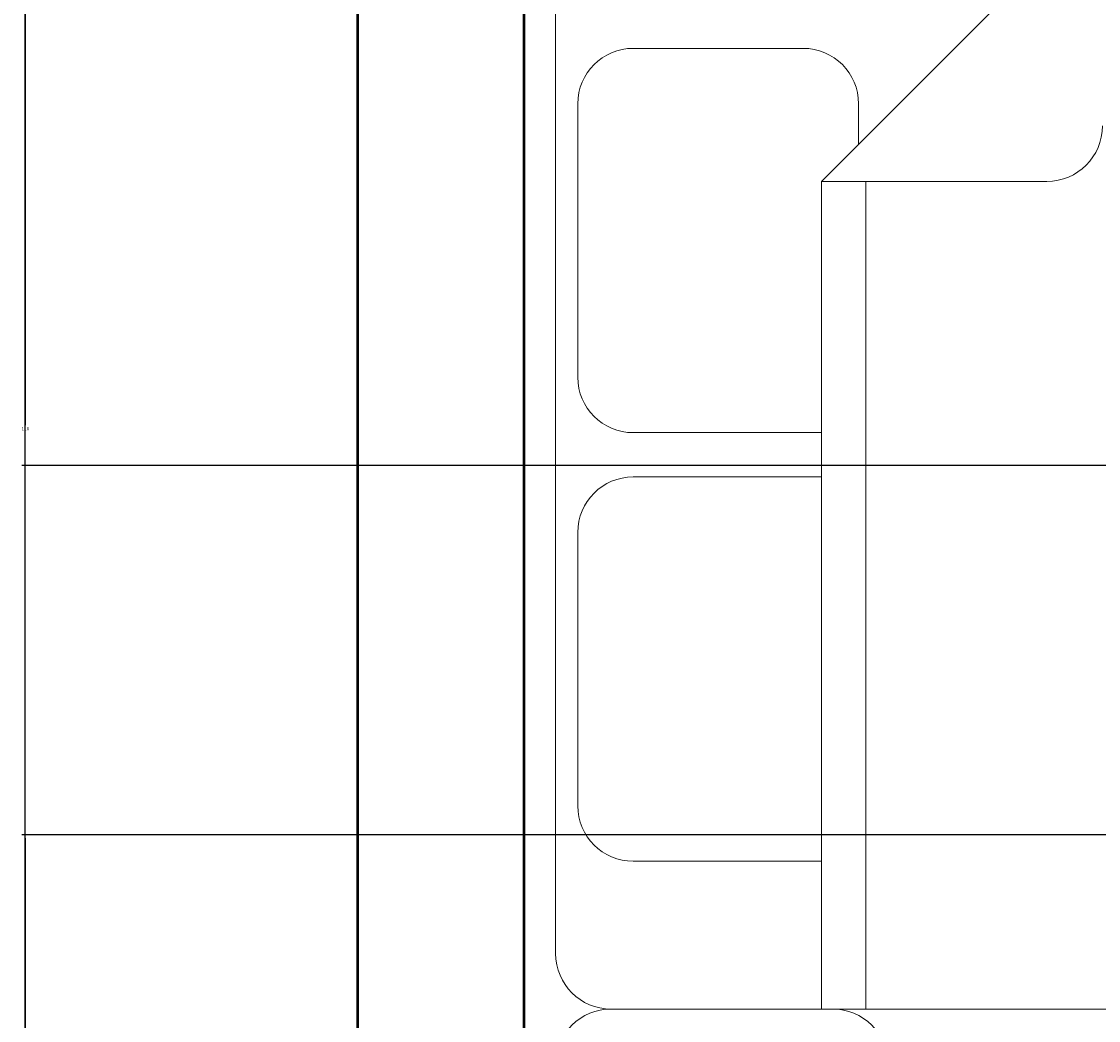
# Model space of a CAD drawing. Units: inches. Extents: x 2621 to 2849, y 2066 to 2463.
# Tile 14 of 28: x 2621 to 2679, y 2345 to 2399. Entities that reach past the tile are written whole.
import ezdxf

# ---------------------------------------------------------------- set-up
doc = ezdxf.new("R2010")
doc.units = ezdxf.units.IN
for name, color, linetype, lineweight in [('A-ANNO-DIMS', 2, 'Continuous', 18), ('A-FURN', 8, 'Continuous', 18), ('A-WALL', 7, 'Continuous', 50)]:
    doc.layers.add(name, color=color, linetype=linetype, lineweight=lineweight)
doc.styles.get("Standard").update_dxf_attribs({"font": 'arial.ttf'})
doc.dimstyles.get("Standard").update_dxf_attribs({"dimtxt": 0.18, "dimasz": 0.18, "dimexe": 0.18, "dimexo": 0.0625, "dimgap": 0.09, "dimtad": 0, "dimtih": 1, "dimtoh": 1, "dimdec": 4, "dimzin": 0, "dimdsep": 46, "dimtxsty": 'Standard', "dimcen": 0.09, "dimadec": 0, "dimazin": 0, "dimtfac": 1, "dimtdec": 4, "dimtofl": 0, "dimtmove": 0, "dimatfit": 3, "dimfxl": 1, "dimtolj": 1, "dimtzin": 0, "dimarcsym": 0})

# ---------------------------------------------------------------- blocks, each defined once
blk = doc.blocks.new('Bed - Queen')
for p, q in [((3, 0), (56.99999, 0)), ((10.99999, -1.2), (25.79998, -1.2)), ((34.19999, -1.2), (48.99999, -1.2)), ((0, -77.00003), (0, -3)), ((7.99999, -14.4), (7.99999, -4.2)), ((28.79998, -4.2), (28.79998, -14.4)), ((31.19999, -14.4), (31.19999, -4.2)), ((51.99999, -4.2), (51.99999, -13.4)), ((0, -14.4), (44.8, -14.4)), ((59.99999, -29.6), (44.8, -14.4)), ((44.8, -14.4), (44.8, -26.6)), ((44.8, -16.8), (0, -16.8)), ((48.99999, -16.4), (46.79936, -16.4))]:
    blk.add_line(p, q)
for centre, start, end in [((3, -3), 90, 180), ((10.99999, -4.2), 90, 180), ((25.79998, -4.2), 0, 90), ((34.19999, -4.2), 90, 180), ((48.99999, -4.2), 0, 90), ((48.99999, -13.4), 270, 0), ((47.8, -26.6), 180, 270)]:
    blk.add_arc(centre, 3, start, end)
blk = doc.blocks.new('*D46')
at = {"layer": 'A-ANNO-DIMS', "color": 0, "lineweight": -2, "transparency": 16777216}
for p, q in [((2647.808, 2435.375), (2620.687, 2435.375)), ((2620.867, 2435.195), (2620.867, 2377.556)), ((2620.867, 2319.555), (2620.867, 2377.193)), ((2647.808, 2319.375), (2620.687, 2319.375))]:
    blk.add_line(p, q, dxfattribs=at)
at = {"layer": 'A-ANNO-DIMS', "color": 0, "transparency": 16777216}
for points in [[(2620.837, 2435.195), (2620.897, 2435.195), (2620.867, 2435.375)], [(2620.837, 2319.555), (2620.897, 2319.555), (2620.867, 2319.375)]]:
    blk.add_solid(points, dxfattribs=at)
at = {"layer": 'Defpoints', "color": 0, "transparency": 16777216}
for p in [(2620.867, 2435.375), (2647.87, 2435.375), (2647.87, 2319.375)]:
    blk.add_point(p, dxfattribs=at)
at = {"layer": 'A-ANNO-DIMS', "color": 0, "transparency": 16777216, "insert": (2620.867, 2377.375), "char_height": 0.18, "attachment_point": 5}
blk.add_mtext('\\A1;116', dxfattribs=at)
blk = doc.blocks.new('*D50')
at = {"layer": 'A-ANNO-DIMS', "color": 0, "lineweight": -2, "transparency": 16777216}
for p, q in [((2763.808, 2355.375), (2620.687, 2355.375)), ((2620.867, 2355.195), (2620.867, 2340.557)), ((2620.867, 2325.555), (2620.867, 2340.193)), ((2763.808, 2325.375), (2620.687, 2325.375))]:
    blk.add_line(p, q, dxfattribs=at)
at = {"layer": 'A-ANNO-DIMS', "color": 0, "transparency": 16777216}
for points in [[(2620.837, 2355.195), (2620.897, 2355.195), (2620.867, 2355.375)], [(2620.837, 2325.555), (2620.897, 2325.555), (2620.867, 2325.375)]]:
    blk.add_solid(points, dxfattribs=at)
at = {"layer": 'Defpoints', "color": 0, "transparency": 16777216}
for p in [(2620.867, 2355.375), (2763.87, 2355.375), (2763.87, 2325.375)]:
    blk.add_point(p, dxfattribs=at)
at = {"layer": 'A-ANNO-DIMS', "color": 0, "transparency": 16777216, "insert": (2620.867, 2340.375), "char_height": 0.18, "attachment_point": 5}
blk.add_mtext('\\A1;30', dxfattribs=at)
blk = doc.blocks.new('*D68')
at = {"layer": 'A-ANNO-DIMS', "color": 0, "lineweight": -2, "transparency": 16777216}
for p, q in [((2745.808, 2435.375), (2620.687, 2435.375)), ((2620.867, 2435.195), (2620.867, 2405.556)), ((2620.867, 2375.555), (2620.867, 2405.193)), ((2745.808, 2375.375), (2620.687, 2375.375))]:
    blk.add_line(p, q, dxfattribs=at)
at = {"layer": 'A-ANNO-DIMS', "color": 0, "transparency": 16777216}
for points in [[(2620.837, 2435.195), (2620.897, 2435.195), (2620.867, 2435.375)], [(2620.837, 2375.555), (2620.897, 2375.555), (2620.867, 2375.375)]]:
    blk.add_solid(points, dxfattribs=at)
at = {"layer": 'Defpoints', "color": 0, "transparency": 16777216}
for p in [(2620.867, 2435.375), (2745.87, 2435.375), (2745.87, 2375.375)]:
    blk.add_point(p, dxfattribs=at)
at = {"layer": 'A-ANNO-DIMS', "color": 0, "transparency": 16777216, "insert": (2620.867, 2405.375), "char_height": 0.18, "attachment_point": 5}
blk.add_mtext('\\A1;60', dxfattribs=at)

msp = doc.modelspace()

# ---------------------------------------------------------------- linework, layer by layer
at = {"layer": 'A-FURN'}
msp.add_lwpolyline([(2652.5811, 2327.9537), (2664.5811, 2327.9537, 0.4142136), (2667.5811, 2330.9537), (2667.5811, 2342.9537, 0.4142136), (2664.5811, 2345.9537), (2652.5811, 2345.9537, 0.4142136), (2649.5811, 2342.9537), (2649.5811, 2330.9537, 0.4142136)], format="xyb", close=True, dxfattribs=at)
at = {"layer": 'A-WALL'}
msp.add_line((2647.8701, 2319.3746), (2647.8701, 2435.3746), dxfattribs=at)
msp.add_lwpolyline([(2761.8701, 2084.3746), (2638.8701, 2084.3746), (2638.8701, 2444.3746), (2830.8701, 2444.3746), (2830.8701, 2084.3746), (2797.8701, 2084.3746)], dxfattribs=at)

# ---------------------------------------------------------------- block references
at = {"layer": 'A-FURN', "rotation": 90}
msp.add_blockref('Bed - Queen', (2649.5811, 2345.9537), dxfattribs=at)

# ---------------------------------------------------------------- dimensions: what is measured, and where the dimension line sits
at = {"layer": 'A-ANNO-DIMS'}
for base, p1, p2, picture, middle in [((2620.8666, 2435.3746), (2647.8701, 2319.3746), (2647.8701, 2435.3746), '*D46', (2620.8666, 2377.3746)), ((2620.8666, 2435.3746), (2745.8701, 2375.3746), (2745.8701, 2435.3746), '*D68', (2620.8666, 2405.3746)), ((2620.8666, 2355.3746), (2763.8701, 2325.3746), (2763.8701, 2355.3746), '*D50', (2620.8666, 2340.3746))]:
    dim = msp.add_linear_dim(base=base, p1=p1, p2=p2, angle=90, dimstyle='Standard', override={"dimdec": 0, "dimlfac": 1, "dimrnd": 0, "dimzin": 0, "dimdsep": 46, "dimlunit": 2}, dxfattribs=at)
    dim.commit()
    dim.dimension.update_dxf_attribs({"geometry": picture, "text_midpoint": middle})

doc.saveas('drawing.dxf')
